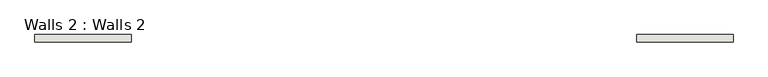
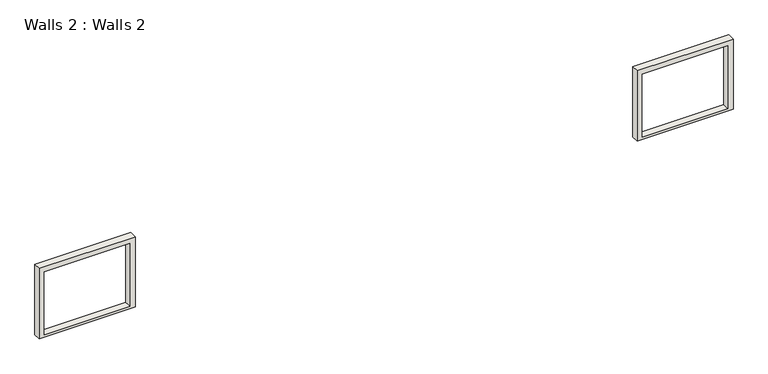
"""IFC4 building model written with IfcOpenShell, lengths in millimetres: wall geometry, Walls 2 : Walls 2."""

from ifc_helpers import new_model, si_unit, frame, origin, place, context, project, spatial, polyline, outline, extrude, source, transform, mapped, element, save


def walls_2_walls_2_bd2c14ef(model_context):
    return source(origin(), model_context, "Body", "SweptSolid", [
        extrude(outline(polyline([(2203.45, -1120.9378119), (2203.45, -2784.6378119), (914.4, -2784.6378119), (914.4, -1120.9378119), (2203.45, -1120.9378119)]), holes=[polyline([(2114.55, -1209.8378119), (954.9188647, -1209.8378119), (954.9188647, -2695.7378119), (2114.55, -2695.7378119), (2114.55, -1209.8378119)])]), frame((0.0, -107.4982733, 0.0), z_axis=(0.0, 1.0, 0.0), x_axis=(0.0, 0.0, 1.0)), (0.0, 0.0, 1.0), 126.5639477),
        extrude(outline(polyline([(2203.45, 9242.2621881), (2203.45, 7578.5621881), (914.4, 7578.5621881), (914.4, 9242.2621881), (2203.45, 9242.2621881)]), holes=[polyline([(2114.55, 9153.3621881), (954.259604, 9153.3621881), (954.259604, 7667.4621881), (2114.55, 7667.4621881), (2114.55, 9153.3621881)])]), frame((0.0, -107.4982733, 0.0), z_axis=(0.0, 1.0, 0.0), x_axis=(0.0, 0.0, 1.0)), (0.0, 0.0, 1.0), 126.5639477),
    ])


if __name__ == "__main__":
    model = new_model("IFC4")
    model_context = context("Model", 3, world=origin())
    ifc_project = project(units=[si_unit("LENGTHUNIT", "METRE", prefix="MILLI")], contexts=[model_context])
    site = spatial("IfcSite", under=ifc_project)
    building = spatial("IfcBuilding", under=site)
    placement = place(None, origin())
    walls_2_walls_2_shape = walls_2_walls_2_bd2c14ef(model_context)
    element("IfcWall", 1, ObjectType="Walls 2 : Walls 2", at=placement, inside=building, context=model_context, shape_type="MappedRepresentation", body=[
        mapped(walls_2_walls_2_shape, transform((0.0, 0.0, 0.0), x_axis=(1.0, 0.0, 0.0), y_axis=(0.0, 1.0, 0.0), z_axis=(0.0, 0.0, 1.0))),
    ])
    save(model, "model.ifc")

# Revit data of these elements
# Element 1 (IfcWall, "Walls 2 : Walls 2")
#   Materials on its faces: "Default Wall"
# Materials
#   "Default Wall": colour RGB 80 80 80, transparency 0
